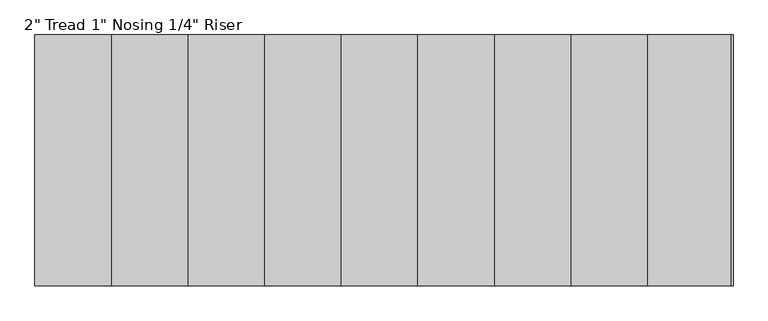
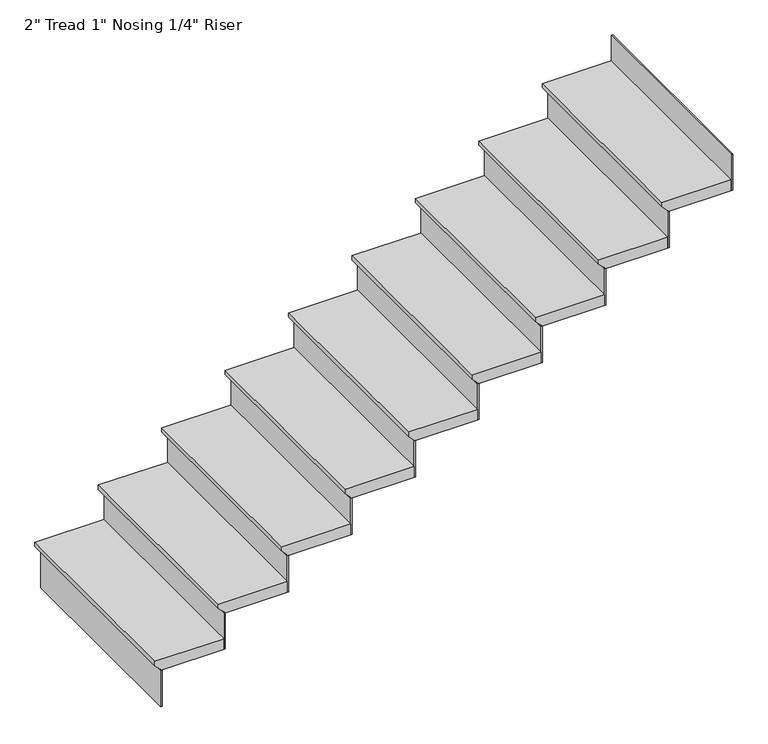
"""IFC4 building model written with IfcOpenShell, lengths in millimetres: stair flight geometry."""

from ifc_helpers import new_model, si_unit, frame, origin, place, context, project, spatial, polyline, outline, extrude, source, transform, mapped, element, save


def stair_flight_d3a95e7b(model_context):
    return source(origin(), model_context, "Body", "SweptSolid", [
        extrude(outline(polyline([(1828.8, -14271.1777023), (1828.8, -14575.9777023), (1809.75, -14575.9777023), (1784.35, -14550.5777023), (1778.0, -14550.5777023), (1778.0, -14271.1777023), (1828.8, -14271.1777023)])), frame((0.0, 788.0679075, 0.0), z_axis=(0.0, 1.0, 0.0), x_axis=(0.0, 0.0, 1.0)), (0.0, 0.0, 1.0), 914.4),
        extrude(outline(polyline([(-14544.2277023, 788.0679075), (-14550.5777023, 788.0679075), (-14550.5777023, 1702.4679075), (-14544.2277023, 1702.4679075), (-14544.2277023, 788.0679075)])), frame((0.0, 0.0, 1608.6666667), z_axis=(0.0, 0.0, 1.0), x_axis=(1.0, 0.0, 0.0)), (0.0, 0.0, 1.0), 169.3333333),
        extrude(outline(polyline([(-14264.8277023, 788.0679075), (-14271.1777023, 788.0679075), (-14271.1777023, 1702.4679075), (-14264.8277023, 1702.4679075), (-14264.8277023, 788.0679075)])), frame((0.0, 0.0, 1778.0), z_axis=(0.0, 0.0, 1.0), x_axis=(1.0, 0.0, 0.0)), (0.0, 0.0, 1.0), 169.3333333),
        extrude(outline(polyline([(1998.1333333, -13991.7777023), (1998.1333333, -14296.5777023), (1979.0833333, -14296.5777023), (1953.6833333, -14271.1777023), (1947.3333333, -14271.1777023), (1947.3333333, -13991.7777023), (1998.1333333, -13991.7777023)])), frame((0.0, 788.0679075, 0.0), z_axis=(0.0, 1.0, 0.0), x_axis=(0.0, 0.0, 1.0)), (0.0, 0.0, 1.0), 914.4),
        extrude(outline(polyline([(-13985.4277023, 788.0679075), (-13991.7777023, 788.0679075), (-13991.7777023, 1702.4679075), (-13985.4277023, 1702.4679075), (-13985.4277023, 788.0679075)])), frame((0.0, 0.0, 1947.3333333), z_axis=(0.0, 0.0, 1.0), x_axis=(1.0, 0.0, 0.0)), (0.0, 0.0, 1.0), 169.3333333),
        extrude(outline(polyline([(2167.4666667, -13712.3777023), (2167.4666667, -14017.1777023), (2148.4166667, -14017.1777023), (2123.0166667, -13991.7777023), (2116.6666667, -13991.7777023), (2116.6666667, -13712.3777023), (2167.4666667, -13712.3777023)])), frame((0.0, 788.0679075, 0.0), z_axis=(0.0, 1.0, 0.0), x_axis=(0.0, 0.0, 1.0)), (0.0, 0.0, 1.0), 914.4),
        extrude(outline(polyline([(-13706.0277023, 788.0679075), (-13712.3777023, 788.0679075), (-13712.3777023, 1702.4679075), (-13706.0277023, 1702.4679075), (-13706.0277023, 788.0679075)])), frame((0.0, 0.0, 2116.6666667), z_axis=(0.0, 0.0, 1.0), x_axis=(1.0, 0.0, 0.0)), (0.0, 0.0, 1.0), 169.3333333),
        extrude(outline(polyline([(2336.8, -13432.9777023), (2336.8, -13737.7777023), (2317.75, -13737.7777023), (2292.35, -13712.3777023), (2286.0, -13712.3777023), (2286.0, -13432.9777023), (2336.8, -13432.9777023)])), frame((0.0, 788.0679075, 0.0), z_axis=(0.0, 1.0, 0.0), x_axis=(0.0, 0.0, 1.0)), (0.0, 0.0, 1.0), 914.4),
        extrude(outline(polyline([(-13426.6277023, 788.0679075), (-13432.9777023, 788.0679075), (-13432.9777023, 1702.4679075), (-13426.6277023, 1702.4679075), (-13426.6277023, 788.0679075)])), frame((0.0, 0.0, 2286.0), z_axis=(0.0, 0.0, 1.0), x_axis=(1.0, 0.0, 0.0)), (0.0, 0.0, 1.0), 169.3333333),
        extrude(outline(polyline([(2506.1333333, -13153.5777023), (2506.1333333, -13458.3777023), (2487.0833333, -13458.3777023), (2461.6833333, -13432.9777023), (2455.3333333, -13432.9777023), (2455.3333333, -13153.5777023), (2506.1333333, -13153.5777023)])), frame((0.0, 788.0679075, 0.0), z_axis=(0.0, 1.0, 0.0), x_axis=(0.0, 0.0, 1.0)), (0.0, 0.0, 1.0), 914.4),
        extrude(outline(polyline([(-13147.2277023, 788.0679075), (-13153.5777023, 788.0679075), (-13153.5777023, 1702.4679075), (-13147.2277023, 1702.4679075), (-13147.2277023, 788.0679075)])), frame((0.0, 0.0, 2455.3333333), z_axis=(0.0, 0.0, 1.0), x_axis=(1.0, 0.0, 0.0)), (0.0, 0.0, 1.0), 169.3333333),
        extrude(outline(polyline([(2675.4666667, -12874.1777023), (2675.4666667, -13178.9777023), (2656.4166667, -13178.9777023), (2631.0166667, -13153.5777023), (2624.6666667, -13153.5777023), (2624.6666667, -12874.1777023), (2675.4666667, -12874.1777023)])), frame((0.0, 788.0679075, 0.0), z_axis=(0.0, 1.0, 0.0), x_axis=(0.0, 0.0, 1.0)), (0.0, 0.0, 1.0), 914.4),
        extrude(outline(polyline([(-12867.8277023, 788.0679075), (-12874.1777023, 788.0679075), (-12874.1777023, 1702.4679075), (-12867.8277023, 1702.4679075), (-12867.8277023, 788.0679075)])), frame((0.0, 0.0, 2624.6666667), z_axis=(0.0, 0.0, 1.0), x_axis=(1.0, 0.0, 0.0)), (0.0, 0.0, 1.0), 169.3333333),
        extrude(outline(polyline([(2844.8, -12594.7777023), (2844.8, -12899.5777023), (2825.75, -12899.5777023), (2800.35, -12874.1777023), (2794.0, -12874.1777023), (2794.0, -12594.7777023), (2844.8, -12594.7777023)])), frame((0.0, 788.0679075, 0.0), z_axis=(0.0, 1.0, 0.0), x_axis=(0.0, 0.0, 1.0)), (0.0, 0.0, 1.0), 914.4),
        extrude(outline(polyline([(-12588.4277023, 788.0679075), (-12594.7777023, 788.0679075), (-12594.7777023, 1702.4679075), (-12588.4277023, 1702.4679075), (-12588.4277023, 788.0679075)])), frame((0.0, 0.0, 2794.0), z_axis=(0.0, 0.0, 1.0), x_axis=(1.0, 0.0, 0.0)), (0.0, 0.0, 1.0), 169.3333333),
        extrude(outline(polyline([(3014.1333333, -12315.3777023), (3014.1333333, -12620.1777023), (2995.0833333, -12620.1777023), (2969.6833333, -12594.7777023), (2963.3333333, -12594.7777023), (2963.3333333, -12315.3777023), (3014.1333333, -12315.3777023)])), frame((0.0, 788.0679075, 0.0), z_axis=(0.0, 1.0, 0.0), x_axis=(0.0, 0.0, 1.0)), (0.0, 0.0, 1.0), 914.4),
        extrude(outline(polyline([(-12309.0277023, 788.0679075), (-12315.3777023, 788.0679075), (-12315.3777023, 1702.4679075), (-12309.0277023, 1702.4679075), (-12309.0277023, 788.0679075)])), frame((0.0, 0.0, 2963.3333333), z_axis=(0.0, 0.0, 1.0), x_axis=(1.0, 0.0, 0.0)), (0.0, 0.0, 1.0), 169.3333333),
        extrude(outline(polyline([(-12029.6277023, 788.0679075), (-12035.9777023, 788.0679075), (-12035.9777023, 1702.4679075), (-12029.6277023, 1702.4679075), (-12029.6277023, 788.0679075)])), frame((0.0, 0.0, 3132.6666667), z_axis=(0.0, 0.0, 1.0), x_axis=(1.0, 0.0, 0.0)), (0.0, 0.0, 1.0), 169.3333333),
        extrude(outline(polyline([(3183.4666667, -12035.9777023), (3183.4666667, -12340.7777023), (3164.4166667, -12340.7777023), (3139.0166667, -12315.3777023), (3132.6666667, -12315.3777023), (3132.6666667, -12035.9777023), (3183.4666667, -12035.9777023)])), frame((0.0, 788.0679075, 0.0), z_axis=(0.0, 1.0, 0.0), x_axis=(0.0, 0.0, 1.0)), (0.0, 0.0, 1.0), 914.4),
    ])


if __name__ == "__main__":
    model = new_model("IFC4")
    model_context = context("Model", 3, world=origin())
    ifc_project = project(units=[si_unit("LENGTHUNIT", "METRE", prefix="MILLI")], contexts=[model_context])
    site = spatial("IfcSite", under=ifc_project)
    building = spatial("IfcBuilding", under=site)
    placement = place(None, origin())
    stair_flight_shape = stair_flight_d3a95e7b(model_context)
    element("IfcStairFlight", 1, ObjectType="2\" Tread 1\" Nosing 1/4\" Riser", at=placement, inside=building, context=model_context, shape_type="MappedRepresentation", body=[
        mapped(stair_flight_shape, transform((0.0, 0.0, 0.0), x_axis=(1.0, 0.0, 0.0), y_axis=(0.0, 1.0, 0.0), z_axis=(0.0, 0.0, 1.0))),
    ])
    save(model, "model.ifc")
